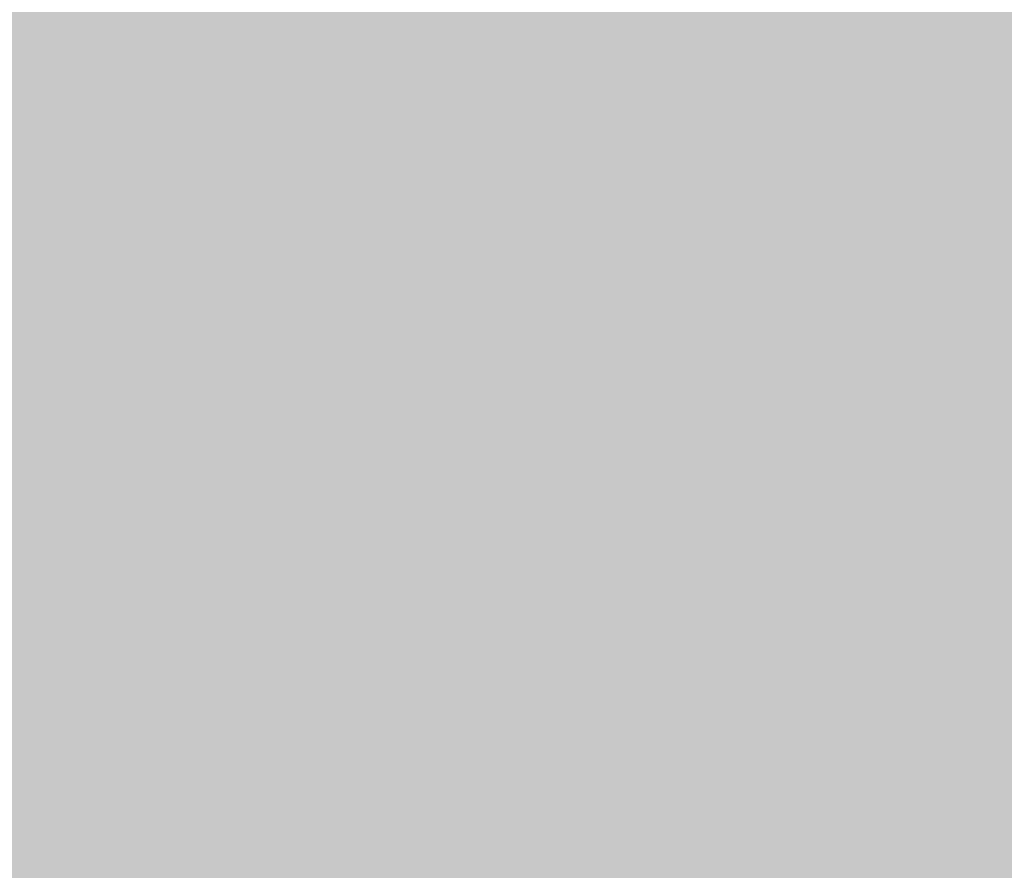
# Model space of a CAD drawing. Units: millimetres. Extents: x -22994 to 29398, y -19990 to 20176.
# Tile 70 of 135: x 225.8137 to 226.3549, y 84.7316 to 85.1994. Entities that reach past the tile are written whole.
import ezdxf
from ezdxf import colors
from ezdxf.entities.mleader import LeaderData, LeaderLine
from ezdxf.math import Vec2, Vec3

# ---------------------------------------------------------------- set-up
doc = ezdxf.new("R2010")
doc.units = ezdxf.units.MM
doc.header["$MEASUREMENT"] = 0
doc.layers.add('M-ANNO-TEXT', color=7, linetype='Continuous', lineweight=25)
doc.layers.add('M-DIMS', color=2, linetype='Continuous', lineweight=18)
doc.styles.get("Standard").update_dxf_attribs({"font": 'arial.ttf'})
doc.dimstyles.get("Standard").update_dxf_attribs({"dimtxt": 0.18, "dimasz": 10000, "dimexe": 0.18, "dimexo": 0.0625, "dimgap": 0.09, "dimtad": 0, "dimtih": 1, "dimtoh": 1, "dimdec": 0, "dimzin": 0, "dimdsep": 46, "dimtxsty": 'Standard', "dimcen": 0.09, "dimadec": 0, "dimazin": 0, "dimtfac": 1, "dimtdec": 0, "dimtofl": 0, "dimtmove": 0, "dimatfit": 3, "dimfxl": 1, "dimtolj": 1, "dimtzin": 0, "dimlwd": 30, "dimarcsym": 0})

# ---------------------------------------------------------------- blocks, each defined once
blk = doc.blocks.new('*D2')
at = {"layer": 'Defpoints', "color": 0, "transparency": 16777216}
for p in [(6.67733, 10.27127), (290.85202, 10.27127), (290.85202, -5.07873)]:
    blk.add_point(p, dxfattribs=at)
at = {"layer": 'M-DIMS', "color": 0, "lineweight": -2, "transparency": 16777216}
for p, q in [((6.67733, 10.20877), (6.67733, -5.25873)), ((290.85202, 10.20877), (290.85202, -5.25873))]:
    blk.add_line(p, q, dxfattribs=at)
at = {"layer": 'M-DIMS', "color": 0, "lineweight": 30, "transparency": 16777216}
for p, q in [((-9993.32267, -5.07873), (-19993.32267, -5.07873)), ((10290.85202, -5.07873), (20290.85202, -5.07873))]:
    blk.add_line(p, q, dxfattribs=at)
at = {"layer": 'M-DIMS', "color": 0, "transparency": 16777216}
for points in [[(-9993.32267, 1661.58794), (-9993.32267, -1671.74539), (6.67733, -5.07873)], [(10290.85202, 1661.58794), (10290.85202, -1671.74539), (290.85202, -5.07873)]]:
    blk.add_solid(points, dxfattribs=at)
at = {"layer": 'M-DIMS', "color": 0, "transparency": 16777216, "insert": (148.76467, -5.07873), "char_height": 0.18, "attachment_point": 5}
blk.add_mtext('\\A1;284.2', dxfattribs=at)
blk = doc.blocks.new('*D3')
at = {"layer": 'Defpoints', "color": 0, "transparency": 16777216}
for p in [(110.26467, 204.16539), (110.26467, 176.36616), (95.83267, 127.96702)]:
    blk.add_point(p, dxfattribs=at)
at = {"layer": 'M-DIMS', "color": 0, "lineweight": -2, "transparency": 16777216}
for p, q in [((95.83267, 128.02952), (95.83267, 204.34539)), ((110.26467, 176.42866), (110.26467, 204.34539))]:
    blk.add_line(p, q, dxfattribs=at)
at = {"layer": 'M-DIMS', "color": 0, "lineweight": 30, "transparency": 16777216}
for p, q in [((-9904.16734, 204.16539), (-19904.16733, 204.16539)), ((10110.26467, 204.16539), (20110.26467, 204.16539))]:
    blk.add_line(p, q, dxfattribs=at)
at = {"layer": 'M-DIMS', "color": 0, "transparency": 16777216}
for points in [[(-9904.16734, 1870.83206), (-9904.16734, -1462.50127), (95.83267, 204.16539)], [(10110.26467, 1870.83206), (10110.26467, -1462.50127), (110.26467, 204.16539)]]:
    blk.add_solid(points, dxfattribs=at)
at = {"layer": 'M-DIMS', "color": 0, "transparency": 16777216, "insert": (103.04867, 204.16539), "char_height": 0.18, "attachment_point": 5}
blk.add_mtext('\\A1;14.432', dxfattribs=at)
blk = doc.blocks.new('*D4')
at = {"layer": 'Defpoints', "color": 0, "transparency": 16777216}
for p in [(116.26467, 204.16539), (110.26467, 176.36616), (116.26467, 176.36616)]:
    blk.add_point(p, dxfattribs=at)
at = {"layer": 'M-DIMS', "color": 0, "lineweight": -2, "transparency": 16777216}
for p, q in [((110.26467, 176.42866), (110.26467, 204.34539)), ((116.26467, 176.42866), (116.26467, 204.34539))]:
    blk.add_line(p, q, dxfattribs=at)
at = {"layer": 'M-DIMS', "color": 0, "lineweight": 30, "transparency": 16777216}
for p, q in [((-9889.73533, 204.16539), (-19889.73533, 204.16539)), ((10116.26467, 204.16539), (20116.26467, 204.16539))]:
    blk.add_line(p, q, dxfattribs=at)
at = {"layer": 'M-DIMS', "color": 0, "transparency": 16777216}
for points in [[(-9889.73533, 1870.83206), (-9889.73533, -1462.50127), (110.26467, 204.16539)], [(10116.26467, 1870.83206), (10116.26467, -1462.50127), (116.26467, 204.16539)]]:
    blk.add_solid(points, dxfattribs=at)
at = {"layer": 'M-DIMS', "color": 0, "transparency": 16777216, "insert": (113.26467, 204.16539), "char_height": 0.18, "attachment_point": 5}
blk.add_mtext('\\A1;6', dxfattribs=at)
blk = doc.blocks.new('*D5')
at = {"layer": 'Defpoints', "color": 0, "transparency": 16777216}
for p in [(181.26467, 204.16539), (116.26467, 176.36616), (181.26467, 176.36616)]:
    blk.add_point(p, dxfattribs=at)
at = {"layer": 'M-DIMS', "color": 0, "lineweight": -2, "transparency": 16777216}
for p, q in [((116.26467, 176.42866), (116.26467, 204.34539)), ((181.26467, 176.42866), (181.26467, 204.34539))]:
    blk.add_line(p, q, dxfattribs=at)
at = {"layer": 'M-DIMS', "color": 0, "lineweight": 30, "transparency": 16777216}
for p, q in [((-9883.73533, 204.16539), (-19883.73533, 204.16539)), ((10181.26467, 204.16539), (20181.26467, 204.16539))]:
    blk.add_line(p, q, dxfattribs=at)
at = {"layer": 'M-DIMS', "color": 0, "transparency": 16777216}
for points in [[(-9883.73533, 1870.83206), (-9883.73533, -1462.50127), (116.26467, 204.16539)], [(10181.26467, 1870.83206), (10181.26467, -1462.50127), (181.26467, 204.16539)]]:
    blk.add_solid(points, dxfattribs=at)
at = {"layer": 'M-DIMS', "color": 0, "transparency": 16777216, "insert": (148.76467, 204.16539), "char_height": 0.18, "attachment_point": 5}
blk.add_mtext('\\A1;65', dxfattribs=at)
blk = doc.blocks.new('*D6')
at = {"layer": 'Defpoints', "color": 0, "transparency": 16777216}
for p in [(187.26467, 204.16539), (181.26467, 176.36616), (187.26467, 176.36616)]:
    blk.add_point(p, dxfattribs=at)
at = {"layer": 'M-DIMS', "color": 0, "lineweight": -2, "transparency": 16777216}
for p, q in [((181.26467, 176.42866), (181.26467, 204.34539)), ((187.26467, 176.42866), (187.26467, 204.34539))]:
    blk.add_line(p, q, dxfattribs=at)
at = {"layer": 'M-DIMS', "color": 0, "lineweight": 30, "transparency": 16777216}
for p, q in [((-9818.73533, 204.16539), (-19818.73533, 204.16539)), ((10187.26467, 204.16539), (20187.26467, 204.16539))]:
    blk.add_line(p, q, dxfattribs=at)
at = {"layer": 'M-DIMS', "color": 0, "transparency": 16777216}
for points in [[(-9818.73533, 1870.83206), (-9818.73533, -1462.50127), (181.26467, 204.16539)], [(10187.26467, 1870.83206), (10187.26467, -1462.50127), (187.26467, 204.16539)]]:
    blk.add_solid(points, dxfattribs=at)
at = {"layer": 'M-DIMS', "color": 0, "transparency": 16777216, "insert": (184.26467, 204.16539), "char_height": 0.18, "attachment_point": 5}
blk.add_mtext('\\A1;6', dxfattribs=at)
blk = doc.blocks.new('*D7')
at = {"layer": 'Defpoints', "color": 0, "transparency": 16777216}
for p in [(201.69668, 204.16539), (187.26467, 176.36616), (201.69668, 127.96702)]:
    blk.add_point(p, dxfattribs=at)
at = {"layer": 'M-DIMS', "color": 0, "lineweight": -2, "transparency": 16777216}
for p, q in [((187.26467, 176.42866), (187.26467, 204.34539)), ((201.69668, 128.02952), (201.69668, 204.34539))]:
    blk.add_line(p, q, dxfattribs=at)
at = {"layer": 'M-DIMS', "color": 0, "lineweight": 30, "transparency": 16777216}
for p, q in [((-9812.73533, 204.16539), (-19812.73533, 204.16539)), ((10201.69668, 204.16539), (20201.69668, 204.16539))]:
    blk.add_line(p, q, dxfattribs=at)
at = {"layer": 'M-DIMS', "color": 0, "transparency": 16777216}
for points in [[(-9812.73533, 1870.83206), (-9812.73533, -1462.50127), (187.26467, 204.16539)], [(10201.69668, 1870.83206), (10201.69668, -1462.50127), (201.69668, 204.16539)]]:
    blk.add_solid(points, dxfattribs=at)
at = {"layer": 'M-DIMS', "color": 0, "transparency": 16777216, "insert": (194.48068, 204.16539), "char_height": 0.18, "attachment_point": 5}
blk.add_mtext('\\A1;14.432', dxfattribs=at)
blk = doc.blocks.new('*D8')
at = {"layer": 'Defpoints', "color": 0, "transparency": 16777216}
for p in [(227.64848, 204.16539), (227.64848, 146.72957), (201.69668, 127.96702)]:
    blk.add_point(p, dxfattribs=at)
at = {"layer": 'M-DIMS', "color": 0, "lineweight": -2, "transparency": 16777216}
for p, q in [((201.69668, 128.02952), (201.69668, 204.34539)), ((227.64848, 146.79207), (227.64848, 204.34539))]:
    blk.add_line(p, q, dxfattribs=at)
at = {"layer": 'M-DIMS', "color": 0, "lineweight": 30, "transparency": 16777216}
for p, q in [((-9798.30332, 204.16539), (-19798.30332, 204.16539)), ((10227.64848, 204.16539), (20227.64848, 204.16539))]:
    blk.add_line(p, q, dxfattribs=at)
at = {"layer": 'M-DIMS', "color": 0, "transparency": 16777216}
for points in [[(-9798.30332, 1870.83206), (-9798.30332, -1462.50127), (201.69668, 204.16539)], [(10227.64848, 1870.83206), (10227.64848, -1462.50127), (227.64848, 204.16539)]]:
    blk.add_solid(points, dxfattribs=at)
at = {"layer": 'M-DIMS', "color": 0, "transparency": 16777216, "insert": (214.67258, 204.16539), "char_height": 0.18, "attachment_point": 5}
blk.add_mtext('\\A1;25.95', dxfattribs=at)
blk = doc.blocks.new('*D9')
at = {"layer": 'Defpoints', "color": 0, "transparency": 16777216}
for p in [(187.26467, 176.36616), (306.20202, 176.36616), (290.85202, 10.27127)]:
    blk.add_point(p, dxfattribs=at)
at = {"layer": 'M-DIMS', "color": 0, "lineweight": 30, "transparency": 16777216}
for p, q in [((306.20202, 10176.36616), (306.20202, 20176.36616)), ((306.20202, -9989.72873), (306.20202, -19989.72873))]:
    blk.add_line(p, q, dxfattribs=at)
at = {"layer": 'M-DIMS', "color": 0, "lineweight": -2, "transparency": 16777216}
for p, q in [((187.32717, 176.36616), (306.38202, 176.36616)), ((290.91452, 10.27127), (306.38202, 10.27127))]:
    blk.add_line(p, q, dxfattribs=at)
at = {"layer": 'M-DIMS', "color": 0, "transparency": 16777216}
for points in [[(-1360.46465, 10176.36616), (1972.86869, 10176.36616), (306.20202, 176.36616)], [(-1360.46465, -9989.72873), (1972.86869, -9989.72873), (306.20202, 10.27127)]]:
    blk.add_solid(points, dxfattribs=at)
at = {"layer": 'M-DIMS', "color": 0, "transparency": 16777216, "insert": (306.20202, 93.31872), "char_height": 0.18, "attachment_point": 5}
blk.add_mtext('\\A1;166.1', dxfattribs=at)
blk = doc.blocks.new('*D10')
at = {"layer": 'Defpoints', "color": 0, "transparency": 16777216}
for p in [(125.64978, 136.0713), (133.34587, 136.0713), (133.34587, -5.07873)]:
    blk.add_point(p, dxfattribs=at)
at = {"layer": 'M-DIMS', "color": 0, "lineweight": -2, "transparency": 16777216}
for p, q in [((125.64978, 136.0088), (125.64978, -5.25872)), ((133.34587, 136.0088), (133.34587, -5.25872))]:
    blk.add_line(p, q, dxfattribs=at)
at = {"layer": 'M-DIMS', "color": 0, "lineweight": 30, "transparency": 16777216}
for p, q in [((-9874.35022, -5.07873), (-19874.35022, -5.07873)), ((10133.34587, -5.07873), (20133.34587, -5.07873))]:
    blk.add_line(p, q, dxfattribs=at)
at = {"layer": 'M-DIMS', "color": 0, "transparency": 16777216}
for points in [[(-9874.35022, 1661.58794), (-9874.35022, -1671.74539), (125.64978, -5.07873)], [(10133.34587, 1661.58794), (10133.34587, -1671.74539), (133.34587, -5.07873)]]:
    blk.add_solid(points, dxfattribs=at)
at = {"layer": 'M-DIMS', "color": 0, "transparency": 16777216, "insert": (129.49783, -5.07873), "char_height": 0.18, "attachment_point": 5}
blk.add_mtext('\\A1;7.696', dxfattribs=at)
blk = doc.blocks.new('*D11')
at = {"layer": 'Defpoints', "color": 0, "transparency": 16777216}
for p in [(133.34587, 136.0713), (135.64978, 136.0713), (135.64978, -5.07873)]:
    blk.add_point(p, dxfattribs=at)
at = {"layer": 'M-DIMS', "color": 0, "lineweight": -2, "transparency": 16777216}
for p, q in [((133.34587, 136.0088), (133.34587, -5.25872)), ((135.64978, 136.0088), (135.64978, -5.25872))]:
    blk.add_line(p, q, dxfattribs=at)
at = {"layer": 'M-DIMS', "color": 0, "lineweight": 30, "transparency": 16777216}
for p, q in [((-9866.65413, -5.07873), (-19866.65413, -5.07873)), ((10135.64978, -5.07873), (20135.64978, -5.07873))]:
    blk.add_line(p, q, dxfattribs=at)
at = {"layer": 'M-DIMS', "color": 0, "transparency": 16777216}
for points in [[(-9866.65413, 1661.58794), (-9866.65413, -1671.74539), (133.34587, -5.07873)], [(10135.64978, 1661.58794), (10135.64978, -1671.74539), (135.64978, -5.07873)]]:
    blk.add_solid(points, dxfattribs=at)
at = {"layer": 'M-DIMS', "color": 0, "transparency": 16777216, "insert": (134.49783, -5.07873), "char_height": 0.18, "attachment_point": 5}
blk.add_mtext('\\A1;2.304', dxfattribs=at)
blk = doc.blocks.new('*D12')
at = {"layer": 'Defpoints', "color": 0, "transparency": 16777216}
for p in [(135.64978, 136.0713), (145.64978, 136.0713), (145.64978, -5.07873)]:
    blk.add_point(p, dxfattribs=at)
at = {"layer": 'M-DIMS', "color": 0, "lineweight": -2, "transparency": 16777216}
for p, q in [((135.64978, 136.0088), (135.64978, -5.25872)), ((145.64978, 136.0088), (145.64978, -5.25872))]:
    blk.add_line(p, q, dxfattribs=at)
at = {"layer": 'M-DIMS', "color": 0, "lineweight": 30, "transparency": 16777216}
for p, q in [((-9864.35022, -5.07873), (-19864.35022, -5.07873)), ((10145.64978, -5.07873), (20145.64978, -5.07873))]:
    blk.add_line(p, q, dxfattribs=at)
at = {"layer": 'M-DIMS', "color": 0, "transparency": 16777216}
for points in [[(-9864.35022, 1661.58794), (-9864.35022, -1671.74539), (135.64978, -5.07873)], [(10145.64978, 1661.58794), (10145.64978, -1671.74539), (145.64978, -5.07873)]]:
    blk.add_solid(points, dxfattribs=at)
at = {"layer": 'M-DIMS', "color": 0, "transparency": 16777216, "insert": (140.64978, -5.07873), "char_height": 0.18, "attachment_point": 5}
blk.add_mtext('\\A1;10', dxfattribs=at)
blk = doc.blocks.new('*D13')
at = {"layer": 'Defpoints', "color": 0, "transparency": 16777216}
for p in [(145.64978, 136.0713), (155.64978, 136.0713), (155.64978, -5.07873)]:
    blk.add_point(p, dxfattribs=at)
at = {"layer": 'M-DIMS', "color": 0, "lineweight": -2, "transparency": 16777216}
for p, q in [((145.64978, 136.0088), (145.64978, -5.25872)), ((155.64978, 136.0088), (155.64978, -5.25872))]:
    blk.add_line(p, q, dxfattribs=at)
at = {"layer": 'M-DIMS', "color": 0, "lineweight": 30, "transparency": 16777216}
for p, q in [((-9854.35022, -5.07873), (-19854.35022, -5.07873)), ((10155.64978, -5.07873), (20155.64978, -5.07873))]:
    blk.add_line(p, q, dxfattribs=at)
at = {"layer": 'M-DIMS', "color": 0, "transparency": 16777216}
for points in [[(-9854.35022, 1661.58794), (-9854.35022, -1671.74539), (145.64978, -5.07873)], [(10155.64978, 1661.58794), (10155.64978, -1671.74539), (155.64978, -5.07873)]]:
    blk.add_solid(points, dxfattribs=at)
at = {"layer": 'M-DIMS', "color": 0, "transparency": 16777216, "insert": (150.64978, -5.07873), "char_height": 0.18, "attachment_point": 5}
blk.add_mtext('\\A1;10', dxfattribs=at)
blk = doc.blocks.new('*D14')
at = {"layer": 'Defpoints', "color": 0, "transparency": 16777216}
for p in [(155.64978, 136.0713), (165.64978, 136.0713), (165.64978, -5.07873)]:
    blk.add_point(p, dxfattribs=at)
at = {"layer": 'M-DIMS', "color": 0, "lineweight": -2, "transparency": 16777216}
for p, q in [((155.64978, 136.0088), (155.64978, -5.25872)), ((165.64978, 136.0088), (165.64978, -5.25872))]:
    blk.add_line(p, q, dxfattribs=at)
at = {"layer": 'M-DIMS', "color": 0, "lineweight": 30, "transparency": 16777216}
for p, q in [((-9844.35022, -5.07873), (-19844.35022, -5.07873)), ((10165.64978, -5.07873), (20165.64978, -5.07873))]:
    blk.add_line(p, q, dxfattribs=at)
at = {"layer": 'M-DIMS', "color": 0, "transparency": 16777216}
for points in [[(-9844.35022, 1661.58794), (-9844.35022, -1671.74539), (155.64978, -5.07873)], [(10165.64978, 1661.58794), (10165.64978, -1671.74539), (165.64978, -5.07873)]]:
    blk.add_solid(points, dxfattribs=at)
at = {"layer": 'M-DIMS', "color": 0, "transparency": 16777216, "insert": (160.64978, -5.07873), "char_height": 0.18, "attachment_point": 5}
blk.add_mtext('\\A1;10', dxfattribs=at)
blk = doc.blocks.new('*D15')
at = {"layer": 'Defpoints', "color": 0, "transparency": 16777216}
for p in [(173.34587, 154.78801), (173.34587, 136.0713), (306.20202, 136.0713)]:
    blk.add_point(p, dxfattribs=at)
at = {"layer": 'M-DIMS', "color": 0, "lineweight": 30, "transparency": 16777216}
for p, q in [((306.20202, 10154.78801), (306.20202, 20154.78801)), ((306.20202, -9863.9287), (306.20202, -19863.9287))]:
    blk.add_line(p, q, dxfattribs=at)
at = {"layer": 'M-DIMS', "color": 0, "lineweight": -2, "transparency": 16777216}
for p, q in [((173.40837, 154.78801), (306.38202, 154.78801)), ((173.40837, 136.0713), (306.38202, 136.0713))]:
    blk.add_line(p, q, dxfattribs=at)
at = {"layer": 'M-DIMS', "color": 0, "transparency": 16777216}
for points in [[(-1360.46465, 10154.78801), (1972.86869, 10154.78801), (306.20202, 154.78801)], [(-1360.46465, -9863.9287), (1972.86869, -9863.9287), (306.20202, 136.0713)]]:
    blk.add_solid(points, dxfattribs=at)
at = {"layer": 'M-DIMS', "color": 0, "transparency": 16777216, "insert": (306.20202, 145.42965), "char_height": 0.18, "attachment_point": 5}
blk.add_mtext('\\A1;18.717', dxfattribs=at)
blk = doc.blocks.new('*D16')
at = {"layer": 'Defpoints', "color": 0, "transparency": 16777216}
for p in [(120.17023, 204.16539), (110.46575, 48.03494), (120.17023, 48.03494)]:
    blk.add_point(p, dxfattribs=at)
at = {"layer": 'M-DIMS', "color": 0, "lineweight": -2, "transparency": 16777216}
for p, q in [((110.46575, 48.09744), (110.46575, 204.34539)), ((120.17023, 48.09744), (120.17023, 204.34539))]:
    blk.add_line(p, q, dxfattribs=at)
at = {"layer": 'M-DIMS', "color": 0, "lineweight": 30, "transparency": 16777216}
for p, q in [((-9889.53425, 204.16539), (-19889.53425, 204.16539)), ((10120.17023, 204.16539), (20120.17023, 204.16539))]:
    blk.add_line(p, q, dxfattribs=at)
at = {"layer": 'M-DIMS', "color": 0, "transparency": 16777216}
for points in [[(-9889.53425, 1870.83206), (-9889.53425, -1462.50127), (110.46575, 204.16539)], [(10120.17023, 1870.83206), (10120.17023, -1462.50127), (120.17023, 204.16539)]]:
    blk.add_solid(points, dxfattribs=at)
at = {"layer": 'M-DIMS', "color": 0, "transparency": 16777216, "insert": (115.31799, 204.16539), "char_height": 0.18, "attachment_point": 5}
blk.add_mtext('\\A1;9.704', dxfattribs=at)
blk = doc.blocks.new('*D17')
at = {"layer": 'Defpoints', "color": 0, "transparency": 16777216}
for p in [(126.17023, 204.16539), (120.17023, 48.03494), (126.17023, 48.03494)]:
    blk.add_point(p, dxfattribs=at)
at = {"layer": 'M-DIMS', "color": 0, "lineweight": -2, "transparency": 16777216}
for p, q in [((120.17023, 48.09744), (120.17023, 204.34539)), ((126.17023, 48.09744), (126.17023, 204.34539))]:
    blk.add_line(p, q, dxfattribs=at)
at = {"layer": 'M-DIMS', "color": 0, "lineweight": 30, "transparency": 16777216}
for p, q in [((-9879.82977, 204.16539), (-19879.82977, 204.16539)), ((10126.17023, 204.16539), (20126.17023, 204.16539))]:
    blk.add_line(p, q, dxfattribs=at)
at = {"layer": 'M-DIMS', "color": 0, "transparency": 16777216}
for points in [[(-9879.82977, 1870.83206), (-9879.82977, -1462.50127), (120.17023, 204.16539)], [(10126.17023, 1870.83206), (10126.17023, -1462.50127), (126.17023, 204.16539)]]:
    blk.add_solid(points, dxfattribs=at)
at = {"layer": 'M-DIMS', "color": 0, "transparency": 16777216, "insert": (123.17023, 204.16539), "char_height": 0.18, "attachment_point": 5}
blk.add_mtext('\\A1;6', dxfattribs=at)
blk = doc.blocks.new('*D18')
at = {"layer": 'Defpoints', "color": 0, "transparency": 16777216}
for p in [(132.17023, 204.16539), (126.17023, 48.03494), (132.17023, 48.03494)]:
    blk.add_point(p, dxfattribs=at)
at = {"layer": 'M-DIMS', "color": 0, "lineweight": -2, "transparency": 16777216}
for p, q in [((126.17023, 48.09744), (126.17023, 204.34539)), ((132.17023, 48.09744), (132.17023, 204.34539))]:
    blk.add_line(p, q, dxfattribs=at)
at = {"layer": 'M-DIMS', "color": 0, "lineweight": 30, "transparency": 16777216}
for p, q in [((-9873.82977, 204.16539), (-19873.82977, 204.16539)), ((10132.17023, 204.16539), (20132.17023, 204.16539))]:
    blk.add_line(p, q, dxfattribs=at)
at = {"layer": 'M-DIMS', "color": 0, "transparency": 16777216}
for points in [[(-9873.82977, 1870.83206), (-9873.82977, -1462.50127), (126.17023, 204.16539)], [(10132.17023, 1870.83206), (10132.17023, -1462.50127), (132.17023, 204.16539)]]:
    blk.add_solid(points, dxfattribs=at)
at = {"layer": 'M-DIMS', "color": 0, "transparency": 16777216, "insert": (129.17023, 204.16539), "char_height": 0.18, "attachment_point": 5}
blk.add_mtext('\\A1;6', dxfattribs=at)
blk = doc.blocks.new('*D19')
at = {"layer": 'Defpoints', "color": 0, "transparency": 16777216}
for p in [(138.17023, 204.16539), (132.17023, 48.03494), (138.17023, 48.03494)]:
    blk.add_point(p, dxfattribs=at)
at = {"layer": 'M-DIMS', "color": 0, "lineweight": -2, "transparency": 16777216}
for p, q in [((132.17023, 48.09744), (132.17023, 204.34539)), ((138.17023, 48.09744), (138.17023, 204.34539))]:
    blk.add_line(p, q, dxfattribs=at)
at = {"layer": 'M-DIMS', "color": 0, "lineweight": 30, "transparency": 16777216}
for p, q in [((-9867.82977, 204.16539), (-19867.82977, 204.16539)), ((10138.17023, 204.16539), (20138.17023, 204.16539))]:
    blk.add_line(p, q, dxfattribs=at)
at = {"layer": 'M-DIMS', "color": 0, "transparency": 16777216}
for points in [[(-9867.82977, 1870.83206), (-9867.82977, -1462.50127), (132.17023, 204.16539)], [(10138.17023, 1870.83206), (10138.17023, -1462.50127), (138.17023, 204.16539)]]:
    blk.add_solid(points, dxfattribs=at)
at = {"layer": 'M-DIMS', "color": 0, "transparency": 16777216, "insert": (135.17023, 204.16539), "char_height": 0.18, "attachment_point": 5}
blk.add_mtext('\\A1;6', dxfattribs=at)
blk = doc.blocks.new('*D20')
at = {"layer": 'Defpoints', "color": 0, "transparency": 16777216}
for p in [(144.17023, 204.16539), (138.17023, 48.03494), (144.17023, 48.03494)]:
    blk.add_point(p, dxfattribs=at)
at = {"layer": 'M-DIMS', "color": 0, "lineweight": -2, "transparency": 16777216}
for p, q in [((138.17023, 48.09744), (138.17023, 204.34539)), ((144.17023, 48.09744), (144.17023, 204.34539))]:
    blk.add_line(p, q, dxfattribs=at)
at = {"layer": 'M-DIMS', "color": 0, "lineweight": 30, "transparency": 16777216}
for p, q in [((-9861.82977, 204.16539), (-19861.82977, 204.16539)), ((10144.17023, 204.16539), (20144.17023, 204.16539))]:
    blk.add_line(p, q, dxfattribs=at)
at = {"layer": 'M-DIMS', "color": 0, "transparency": 16777216}
for points in [[(-9861.82977, 1870.83206), (-9861.82977, -1462.50127), (138.17023, 204.16539)], [(10144.17023, 1870.83206), (10144.17023, -1462.50127), (144.17023, 204.16539)]]:
    blk.add_solid(points, dxfattribs=at)
at = {"layer": 'M-DIMS', "color": 0, "transparency": 16777216, "insert": (141.17023, 204.16539), "char_height": 0.18, "attachment_point": 5}
blk.add_mtext('\\A1;6', dxfattribs=at)
blk = doc.blocks.new('*D21')
at = {"layer": 'Defpoints', "color": 0, "transparency": 16777216}
for p in [(149.11567, 204.16539), (144.17023, 48.03494), (149.11567, 48.03494)]:
    blk.add_point(p, dxfattribs=at)
at = {"layer": 'M-DIMS', "color": 0, "lineweight": -2, "transparency": 16777216}
for p, q in [((144.17023, 48.09744), (144.17023, 204.34539)), ((149.11567, 48.09744), (149.11567, 204.34539))]:
    blk.add_line(p, q, dxfattribs=at)
at = {"layer": 'M-DIMS', "color": 0, "lineweight": 30, "transparency": 16777216}
for p, q in [((-9855.82977, 204.16539), (-19855.82977, 204.16539)), ((10149.11567, 204.16539), (20149.11567, 204.16539))]:
    blk.add_line(p, q, dxfattribs=at)
at = {"layer": 'M-DIMS', "color": 0, "transparency": 16777216}
for points in [[(-9855.82977, 1870.83206), (-9855.82977, -1462.50127), (144.17023, 204.16539)], [(10149.11567, 1870.83206), (10149.11567, -1462.50127), (149.11567, 204.16539)]]:
    blk.add_solid(points, dxfattribs=at)
at = {"layer": 'M-DIMS', "color": 0, "transparency": 16777216, "insert": (146.64295, 204.16539), "char_height": 0.18, "attachment_point": 5}
blk.add_mtext('\\A1;4.945', dxfattribs=at)
blk = doc.blocks.new('*D22')
at = {"layer": 'Defpoints', "color": 0, "transparency": 16777216}
for p in [(149.11567, 30.98952), (155.11567, 30.98952), (155.11567, -5.07873)]:
    blk.add_point(p, dxfattribs=at)
at = {"layer": 'M-DIMS', "color": 0, "lineweight": -2, "transparency": 16777216}
for p, q in [((149.11567, 30.92702), (149.11567, -5.25872)), ((155.11567, 30.92702), (155.11567, -5.25872))]:
    blk.add_line(p, q, dxfattribs=at)
at = {"layer": 'M-DIMS', "color": 0, "lineweight": 30, "transparency": 16777216}
for p, q in [((-9850.88433, -5.07873), (-19850.88433, -5.07873)), ((10155.11567, -5.07873), (20155.11567, -5.07873))]:
    blk.add_line(p, q, dxfattribs=at)
at = {"layer": 'M-DIMS', "color": 0, "transparency": 16777216}
for points in [[(-9850.88433, 1661.58794), (-9850.88433, -1671.74539), (149.11567, -5.07873)], [(10155.11567, 1661.58794), (10155.11567, -1671.74539), (155.11567, -5.07873)]]:
    blk.add_solid(points, dxfattribs=at)
at = {"layer": 'M-DIMS', "color": 0, "transparency": 16777216, "insert": (152.11567, -5.07873), "char_height": 0.18, "attachment_point": 5}
blk.add_mtext('\\A1;6', dxfattribs=at)
blk = doc.blocks.new('*D23')
at = {"layer": 'Defpoints', "color": 0, "transparency": 16777216}
for p in [(155.11567, 30.98952), (161.11567, 30.98952), (161.11567, -5.07873)]:
    blk.add_point(p, dxfattribs=at)
at = {"layer": 'M-DIMS', "color": 0, "lineweight": -2, "transparency": 16777216}
for p, q in [((155.11567, 30.92702), (155.11567, -5.25872)), ((161.11567, 30.92702), (161.11567, -5.25872))]:
    blk.add_line(p, q, dxfattribs=at)
at = {"layer": 'M-DIMS', "color": 0, "lineweight": 30, "transparency": 16777216}
for p, q in [((-9844.88433, -5.07873), (-19844.88433, -5.07873)), ((10161.11567, -5.07873), (20161.11567, -5.07873))]:
    blk.add_line(p, q, dxfattribs=at)
at = {"layer": 'M-DIMS', "color": 0, "transparency": 16777216}
for points in [[(-9844.88433, 1661.58794), (-9844.88433, -1671.74539), (155.11567, -5.07873)], [(10161.11567, 1661.58794), (10161.11567, -1671.74539), (161.11567, -5.07873)]]:
    blk.add_solid(points, dxfattribs=at)
at = {"layer": 'M-DIMS', "color": 0, "transparency": 16777216, "insert": (158.11567, -5.07873), "char_height": 0.18, "attachment_point": 5}
blk.add_mtext('\\A1;6', dxfattribs=at)
blk = doc.blocks.new('*D24')
at = {"layer": 'Defpoints', "color": 0, "transparency": 16777216}
for p in [(161.11567, 30.98952), (166.43874, 30.98952), (166.43874, -5.07873)]:
    blk.add_point(p, dxfattribs=at)
at = {"layer": 'M-DIMS', "color": 0, "lineweight": -2, "transparency": 16777216}
for p, q in [((161.11567, 30.92702), (161.11567, -5.25872)), ((166.43874, 30.92702), (166.43874, -5.25872))]:
    blk.add_line(p, q, dxfattribs=at)
at = {"layer": 'M-DIMS', "color": 0, "lineweight": 30, "transparency": 16777216}
for p, q in [((-9838.88433, -5.07873), (-19838.88433, -5.07873)), ((10166.43874, -5.07873), (20166.43874, -5.07873))]:
    blk.add_line(p, q, dxfattribs=at)
at = {"layer": 'M-DIMS', "color": 0, "transparency": 16777216}
for points in [[(-9838.88433, 1661.58794), (-9838.88433, -1671.74539), (161.11567, -5.07873)], [(10166.43874, 1661.58794), (10166.43874, -1671.74539), (166.43874, -5.07873)]]:
    blk.add_solid(points, dxfattribs=at)
at = {"layer": 'M-DIMS', "color": 0, "transparency": 16777216, "insert": (163.7772, -5.07873), "char_height": 0.18, "attachment_point": 5}
blk.add_mtext('\\A1;5.323', dxfattribs=at)
blk = doc.blocks.new('*D25')
at = {"layer": 'Defpoints', "color": 0, "transparency": 16777216}
for p in [(166.43874, 30.98952), (172.43874, 30.98952), (172.43874, -5.07873)]:
    blk.add_point(p, dxfattribs=at)
at = {"layer": 'M-DIMS', "color": 0, "lineweight": -2, "transparency": 16777216}
for p, q in [((166.43874, 30.92702), (166.43874, -5.25872)), ((172.43874, 30.92702), (172.43874, -5.25872))]:
    blk.add_line(p, q, dxfattribs=at)
at = {"layer": 'M-DIMS', "color": 0, "lineweight": 30, "transparency": 16777216}
for p, q in [((-9833.56126, -5.07873), (-19833.56126, -5.07873)), ((10172.43874, -5.07873), (20172.43874, -5.07873))]:
    blk.add_line(p, q, dxfattribs=at)
at = {"layer": 'M-DIMS', "color": 0, "transparency": 16777216}
for points in [[(-9833.56126, 1661.58794), (-9833.56126, -1671.74539), (166.43874, -5.07873)], [(10172.43874, 1661.58794), (10172.43874, -1671.74539), (172.43874, -5.07873)]]:
    blk.add_solid(points, dxfattribs=at)
at = {"layer": 'M-DIMS', "color": 0, "transparency": 16777216, "insert": (169.43874, -5.07873), "char_height": 0.18, "attachment_point": 5}
blk.add_mtext('\\A1;6', dxfattribs=at)
blk = doc.blocks.new('*D26')
at = {"layer": 'Defpoints', "color": 0, "transparency": 16777216}
for p in [(172.43874, 30.98952), (178.43874, 30.98952), (178.43874, -5.07873)]:
    blk.add_point(p, dxfattribs=at)
at = {"layer": 'M-DIMS', "color": 0, "lineweight": -2, "transparency": 16777216}
for p, q in [((172.43874, 30.92702), (172.43874, -5.25872)), ((178.43874, 30.92702), (178.43874, -5.25872))]:
    blk.add_line(p, q, dxfattribs=at)
at = {"layer": 'M-DIMS', "color": 0, "lineweight": 30, "transparency": 16777216}
for p, q in [((-9827.56126, -5.07873), (-19827.56126, -5.07873)), ((10178.43874, -5.07873), (20178.43874, -5.07873))]:
    blk.add_line(p, q, dxfattribs=at)
at = {"layer": 'M-DIMS', "color": 0, "transparency": 16777216}
for points in [[(-9827.56126, 1661.58794), (-9827.56126, -1671.74539), (172.43874, -5.07873)], [(10178.43874, 1661.58794), (10178.43874, -1671.74539), (178.43874, -5.07873)]]:
    blk.add_solid(points, dxfattribs=at)
at = {"layer": 'M-DIMS', "color": 0, "transparency": 16777216, "insert": (175.43874, -5.07873), "char_height": 0.18, "attachment_point": 5}
blk.add_mtext('\\A1;6', dxfattribs=at)
blk = doc.blocks.new('*D27')
at = {"layer": 'Defpoints', "color": 0, "transparency": 16777216}
for p in [(178.43874, 30.98952), (188.11747, 30.98952), (188.11747, -5.07873)]:
    blk.add_point(p, dxfattribs=at)
at = {"layer": 'M-DIMS', "color": 0, "lineweight": -2, "transparency": 16777216}
for p, q in [((178.43874, 30.92702), (178.43874, -5.25872)), ((188.11747, 30.92702), (188.11747, -5.25872))]:
    blk.add_line(p, q, dxfattribs=at)
at = {"layer": 'M-DIMS', "color": 0, "lineweight": 30, "transparency": 16777216}
for p, q in [((-9821.56126, -5.07873), (-19821.56126, -5.07873)), ((10188.11747, -5.07873), (20188.11747, -5.07873))]:
    blk.add_line(p, q, dxfattribs=at)
at = {"layer": 'M-DIMS', "color": 0, "transparency": 16777216}
for points in [[(-9821.56126, 1661.58794), (-9821.56126, -1671.74539), (178.43874, -5.07873)], [(10188.11747, 1661.58794), (10188.11747, -1671.74539), (188.11747, -5.07873)]]:
    blk.add_solid(points, dxfattribs=at)
at = {"layer": 'M-DIMS', "color": 0, "transparency": 16777216, "insert": (183.27811, -5.07873), "char_height": 0.18, "attachment_point": 5}
blk.add_mtext('\\A1;9.679', dxfattribs=at)
blk = doc.blocks.new('*D28')
at = {"layer": 'Defpoints', "color": 0, "transparency": 16777216}
for p in [(188.11747, 48.03494), (306.20202, 48.03494), (188.11747, 30.98952)]:
    blk.add_point(p, dxfattribs=at)
at = {"layer": 'M-DIMS', "color": 0, "lineweight": 30, "transparency": 16777216}
for p, q in [((306.20202, 10048.03494), (306.20202, 20048.03494)), ((306.20202, -9969.01048), (306.20202, -19969.01048))]:
    blk.add_line(p, q, dxfattribs=at)
at = {"layer": 'M-DIMS', "color": 0, "lineweight": -2, "transparency": 16777216}
for p, q in [((188.17997, 48.03494), (306.38202, 48.03494)), ((188.17997, 30.98952), (306.38202, 30.98952))]:
    blk.add_line(p, q, dxfattribs=at)
at = {"layer": 'M-DIMS', "color": 0, "transparency": 16777216}
for points in [[(-1360.46465, 10048.03494), (1972.86869, 10048.03494), (306.20202, 48.03494)], [(-1360.46465, -9969.01048), (1972.86869, -9969.01048), (306.20202, 30.98952)]]:
    blk.add_solid(points, dxfattribs=at)
at = {"layer": 'M-DIMS', "color": 0, "transparency": 16777216, "insert": (306.20202, 39.51223), "char_height": 0.18, "attachment_point": 5}
blk.add_mtext('\\A1;17.045', dxfattribs=at)
blk = doc.blocks.new('*D29')
at = {"layer": 'Defpoints', "color": 0, "transparency": 16777216}
for p in [(36.80064, 80.04502), (64.02964, 80.045)]:
    blk.add_point(p, dxfattribs=at)
at = {"layer": 'M-DIMS', "color": 0, "lineweight": -2, "transparency": 16777216}
for p, q in [((50.41514, 79.95501), (50.41514, 80.13501)), ((50.32514, 80.04501), (50.50514, 80.04501))]:
    blk.add_line(p, q, dxfattribs=at)
at = {"layer": 'M-DIMS', "color": 0, "lineweight": 30, "transparency": 16777216}
blk.add_line((20064.02964, 80.03031), (10064.02964, 80.03765), dxfattribs=at)
at = {"layer": 'M-DIMS', "color": 0, "transparency": 16777216}
blk.add_solid([(10064.03087, 1746.70432), (10064.02842, -1586.62901), (64.02964, 80.045)], dxfattribs=at)
at = {"layer": 'M-DIMS', "color": 0, "transparency": 16777216, "insert": (20064.52126, 80.03031), "char_height": 0.18, "attachment_point": 5}
blk.add_mtext('\\A1;∅27.23', dxfattribs=at)
blk = doc.blocks.new('*D30')
at = {"layer": 'Defpoints', "color": 0, "transparency": 16777216}
for p in [(216.31485, 146.72913), (238.98211, 146.73)]:
    blk.add_point(p, dxfattribs=at)
at = {"layer": 'M-DIMS', "color": 0, "lineweight": 30, "transparency": 16777216}
blk.add_line((20238.9821, 147.49586), (10238.98211, 147.11293), dxfattribs=at)
at = {"layer": 'M-DIMS', "color": 0, "lineweight": -2, "transparency": 16777216}
for p, q in [((227.64848, 146.63957), (227.64848, 146.81957)), ((227.55848, 146.72957), (227.73848, 146.72957))]:
    blk.add_line(p, q, dxfattribs=at)
at = {"layer": 'M-DIMS', "color": 0, "transparency": 16777216}
blk.add_solid([(10238.91828, 1813.7796), (10239.04593, -1519.55373), (238.98211, 146.73)], dxfattribs=at)
at = {"layer": 'M-DIMS', "color": 0, "transparency": 16777216, "insert": (20239.54365, 147.49586), "char_height": 0.18, "attachment_point": 5}
blk.add_mtext('\\A1;∅22.667', dxfattribs=at)
blk = doc.blocks.new('*D31')
at = {"layer": 'Defpoints', "color": 0, "transparency": 16777216}
for p in [(223.16413, 146.72913), (232.13283, 146.73)]:
    blk.add_point(p, dxfattribs=at)
at = {"layer": 'M-DIMS', "color": 0, "lineweight": 30, "transparency": 16777216}
blk.add_line((20232.13273, 148.66562), (10232.13278, 147.69781), dxfattribs=at)
at = {"layer": 'M-DIMS', "color": 0, "lineweight": -2, "transparency": 16777216}
for p, q in [((227.64848, 146.63957), (227.64848, 146.81957)), ((227.55848, 146.72957), (227.73848, 146.72957))]:
    blk.add_line(p, q, dxfattribs=at)
at = {"layer": 'M-DIMS', "color": 0, "transparency": 16777216}
blk.add_solid([(10231.97148, 1814.36447), (10232.29408, -1518.96885), (232.13283, 146.73)], dxfattribs=at)
at = {"layer": 'M-DIMS', "color": 0, "transparency": 16777216, "insert": (20232.62454, 148.66562), "char_height": 0.18, "attachment_point": 5}
blk.add_mtext('\\A1;∅8.969', dxfattribs=at)
blk = doc.blocks.new('*D36')
at = {"layer": 'Defpoints', "color": 0, "transparency": 16777216}
for p in [(46.39, 31.30349), (46.38747, 26.59341)]:
    blk.add_point(p, dxfattribs=at)
at = {"layer": 'M-DIMS', "color": 0, "lineweight": 30, "transparency": 16777216}
for p, q in [((57.1499, 20031.3006), (51.76995, 10031.30205)), ((10057.1499, 20031.3006), (57.1499, 20031.3006))]:
    blk.add_line(p, q, dxfattribs=at)
at = {"layer": 'M-DIMS', "color": 0, "lineweight": -2, "transparency": 16777216}
for p, q in [((46.38873, 28.85845), (46.38873, 29.03845)), ((46.29873, 28.94845), (46.47873, 28.94845))]:
    blk.add_line(p, q, dxfattribs=at)
at = {"layer": 'M-DIMS', "color": 0, "transparency": 16777216}
blk.add_solid([(-1614.89648, 10032.1987), (1718.43638, 10030.40539), (46.39, 31.30349)], dxfattribs=at)
at = {"layer": 'M-DIMS', "color": 0, "transparency": 16777216, "insert": (10057.55422, 20031.3006), "char_height": 0.18, "attachment_point": 5}
blk.add_mtext('\\A1;∅4.71', dxfattribs=at)

msp = doc.modelspace()

# ---------------------------------------------------------------- dimensions: what is measured, and where the dimension line sits
at = {"layer": 'M-DIMS'}
for base, p1, p2, override, picture, middle in [((306.20202, 176.36616), (290.85202, 10.27127), (187.26467, 176.36616), {"dimdec": 1, "dimlfac": 1, "dimrnd": 0, "dimzin": 0, "dimdsep": 46, "dimlunit": 2}, '*D9', (306.20202, 93.31872)), ((306.20202, 136.0713), (173.34587, 154.78801), (173.34587, 136.0713), {"dimdec": 3, "dimlfac": 1, "dimrnd": 0, "dimzin": 0, "dimdsep": 46, "dimlunit": 2}, '*D15', (306.20202, 145.42965)), ((306.20202, 48.03494), (188.11747, 30.98952), (188.11747, 48.03494), {"dimdec": 3, "dimlfac": 1, "dimrnd": 0, "dimzin": 0, "dimdsep": 46, "dimlunit": 2}, '*D28', (306.20202, 39.51223))]:
    dim = msp.add_linear_dim(base=base, p1=p1, p2=p2, angle=90, dimstyle='Standard', override=override, dxfattribs=at)
    dim.commit()
    dim.dimension.update_dxf_attribs({"geometry": picture, "text_midpoint": middle})
for p1, p2, override, picture, middle in [((46.38747, 26.59341), (46.39, 31.30349), {"dimdec": 2, "dimlfac": 1, "dimrnd": 0, "dimzin": 0, "dimdsep": 46, "dimlunit": 2}, '*D36', (10057.55422, 20031.3006)), ((223.16413, 146.72913), (232.13283, 146.73), {"dimdec": 3, "dimlfac": 1, "dimrnd": 0, "dimzin": 0, "dimdsep": 46, "dimlunit": 2}, '*D31', (20232.13273, 148.66562)), ((216.31485, 146.72913), (238.98211, 146.73), {"dimdec": 3, "dimlfac": 1, "dimrnd": 0, "dimzin": 0, "dimdsep": 46, "dimlunit": 2}, '*D30', (20238.9821, 147.49586))]:
    dim = msp.add_diameter_dim_2p(p1=p1, p2=p2, dimstyle='Standard', override=override, dxfattribs=at)
    dim.commit()
    dim.dimension.update_dxf_attribs({"geometry": picture, "text_midpoint": middle, "dimtype": 163})
for base, p1, p2, override, picture, middle in [((110.26467, 204.16539), (95.83267, 127.96702), (110.26467, 176.36616), {"dimdec": 3, "dimlfac": 1, "dimrnd": 0, "dimzin": 0, "dimdsep": 46, "dimlunit": 2}, '*D3', (103.04867, 204.16539)), ((116.26467, 204.16539), (110.26467, 176.36616), (116.26467, 176.36616), {"dimdec": 0, "dimlfac": 1, "dimrnd": 0, "dimzin": 0, "dimdsep": 46, "dimlunit": 2}, '*D4', (113.26467, 204.16539)), ((120.17023, 204.16539), (110.46575, 48.03494), (120.17023, 48.03494), {"dimdec": 3, "dimlfac": 1, "dimrnd": 0, "dimzin": 0, "dimdsep": 46, "dimlunit": 2}, '*D16', (115.31799, 204.16539)), ((181.26467, 204.16539), (116.26467, 176.36616), (181.26467, 176.36616), {"dimdec": 0, "dimlfac": 1, "dimrnd": 0, "dimzin": 0, "dimdsep": 46, "dimlunit": 2}, '*D5', (148.76467, 204.16539)), ((126.17023, 204.16539), (120.17023, 48.03494), (126.17023, 48.03494), {"dimdec": 0, "dimlfac": 1, "dimrnd": 0, "dimzin": 0, "dimdsep": 46, "dimlunit": 2}, '*D17', (123.17023, 204.16539)), ((132.17023, 204.16539), (126.17023, 48.03494), (132.17023, 48.03494), {"dimdec": 0, "dimlfac": 1, "dimrnd": 0, "dimzin": 0, "dimdsep": 46, "dimlunit": 2}, '*D18', (129.17023, 204.16539)), ((138.17023, 204.16539), (132.17023, 48.03494), (138.17023, 48.03494), {"dimdec": 0, "dimlfac": 1, "dimrnd": 0, "dimzin": 0, "dimdsep": 46, "dimlunit": 2}, '*D19', (135.17023, 204.16539)), ((144.17023, 204.16539), (138.17023, 48.03494), (144.17023, 48.03494), {"dimdec": 0, "dimlfac": 1, "dimrnd": 0, "dimzin": 0, "dimdsep": 46, "dimlunit": 2}, '*D20', (141.17023, 204.16539)), ((149.11567, 204.16539), (144.17023, 48.03494), (149.11567, 48.03494), {"dimdec": 3, "dimlfac": 1, "dimrnd": 0, "dimzin": 0, "dimdsep": 46, "dimlunit": 2}, '*D21', (146.64295, 204.16539)), ((187.26467, 204.16539), (181.26467, 176.36616), (187.26467, 176.36616), {"dimdec": 0, "dimlfac": 1, "dimrnd": 0, "dimzin": 0, "dimdsep": 46, "dimlunit": 2}, '*D6', (184.26467, 204.16539)), ((201.69668, 204.16539), (187.26467, 176.36616), (201.69668, 127.96702), {"dimdec": 3, "dimlfac": 1, "dimrnd": 0, "dimzin": 0, "dimdsep": 46, "dimlunit": 2}, '*D7', (194.48068, 204.16539)), ((227.64848, 204.16539), (201.69668, 127.96702), (227.64848, 146.72957), {"dimdec": 2, "dimlfac": 1, "dimrnd": 0, "dimzin": 0, "dimdsep": 46, "dimlunit": 2}, '*D8', (214.67258, 204.16539)), ((290.85202, -5.07873), (6.67733, 10.27127), (290.85202, 10.27127), {"dimdec": 1, "dimlfac": 1, "dimrnd": 0, "dimzin": 0, "dimdsep": 46, "dimlunit": 2}, '*D2', (148.76467, -5.07873)), ((133.34587, -5.07873), (125.64978, 136.0713), (133.34587, 136.0713), {"dimdec": 3, "dimlfac": 1, "dimrnd": 0, "dimzin": 0, "dimdsep": 46, "dimlunit": 2}, '*D10', (129.49783, -5.07873)), ((135.64978, -5.07873), (133.34587, 136.0713), (135.64978, 136.0713), {"dimdec": 3, "dimlfac": 1, "dimrnd": 0, "dimzin": 0, "dimdsep": 46, "dimlunit": 2}, '*D11', (134.49783, -5.07873)), ((145.64978, -5.07873), (135.64978, 136.0713), (145.64978, 136.0713), {"dimdec": 0, "dimlfac": 1, "dimrnd": 0, "dimzin": 0, "dimdsep": 46, "dimlunit": 2}, '*D12', (140.64978, -5.07873)), ((155.64978, -5.07873), (145.64978, 136.0713), (155.64978, 136.0713), {"dimdec": 0, "dimlfac": 1, "dimrnd": 0, "dimzin": 0, "dimdsep": 46, "dimlunit": 2}, '*D13', (150.64978, -5.07873)), ((155.11567, -5.07873), (149.11567, 30.98952), (155.11567, 30.98952), {"dimdec": 0, "dimlfac": 1, "dimrnd": 0, "dimzin": 0, "dimdsep": 46, "dimlunit": 2}, '*D22', (152.11567, -5.07873)), ((161.11567, -5.07873), (155.11567, 30.98952), (161.11567, 30.98952), {"dimdec": 0, "dimlfac": 1, "dimrnd": 0, "dimzin": 0, "dimdsep": 46, "dimlunit": 2}, '*D23', (158.11567, -5.07873)), ((165.64978, -5.07873), (155.64978, 136.0713), (165.64978, 136.0713), {"dimdec": 0, "dimlfac": 1, "dimrnd": 0, "dimzin": 0, "dimdsep": 46, "dimlunit": 2}, '*D14', (160.64978, -5.07873)), ((166.43874, -5.07873), (161.11567, 30.98952), (166.43874, 30.98952), {"dimdec": 3, "dimlfac": 1, "dimrnd": 0, "dimzin": 0, "dimdsep": 46, "dimlunit": 2}, '*D24', (163.7772, -5.07873)), ((172.43874, -5.07873), (166.43874, 30.98952), (172.43874, 30.98952), {"dimdec": 0, "dimlfac": 1, "dimrnd": 0, "dimzin": 0, "dimdsep": 46, "dimlunit": 2}, '*D25', (169.43874, -5.07873)), ((178.43874, -5.07873), (172.43874, 30.98952), (178.43874, 30.98952), {"dimdec": 0, "dimlfac": 1, "dimrnd": 0, "dimzin": 0, "dimdsep": 46, "dimlunit": 2}, '*D26', (175.43874, -5.07873)), ((188.11747, -5.07873), (178.43874, 30.98952), (188.11747, 30.98952), {"dimdec": 3, "dimlfac": 1, "dimrnd": 0, "dimzin": 0, "dimdsep": 46, "dimlunit": 2}, '*D27', (183.27811, -5.07873))]:
    dim = msp.add_linear_dim(base=base, p1=p1, p2=p2, dimstyle='Standard', override=override, dxfattribs=at)
    dim.commit()
    dim.dimension.update_dxf_attribs({"geometry": picture, "text_midpoint": middle})
dim = msp.add_diameter_dim_2p(p1=(36.80064, 80.04502), p2=(64.02964, 80.045), dimstyle='Standard', override={"dimdec": 2, "dimlfac": 1, "dimrnd": 0, "dimzin": 0, "dimdsep": 46, "dimlunit": 2}, dxfattribs=at)
dim.commit()
dim.dimension.update_dxf_attribs({"geometry": '*D29', "text_midpoint": (20064.02964, 80.03031)})

# ---------------------------------------------------------------- leaders
at = {"layer": 'M-ANNO-TEXT'}
ml = msp.add_multileader_mtext('Standard', dxfattribs=at)
ml.set_content('combustion chamber', color=256)
ml.set_leader_properties()
ml.build(insert=Vec2(0, 0))
ml.multileader.update_dxf_attribs({"dogleg_length": 0.36, "arrow_head_size": 200})
ctx = ml.context
ctx.base_point, ctx.char_height, ctx.arrow_head_size, ctx.landing_gap_size, ctx.plane_origin = Vec3(215.73207, 57.91489), 3, 200, 0.09, Vec3(189.11747, 57.91489)
notes = []
notes.append((ctx, [(0, (1, 1, 0), (215.37207, 57.91489), (1, 0), 0.36, [(0, [(189.11747, 57.91489)], 0, [])])]))
ctx.mtext.insert, ctx.mtext.flow_direction = Vec3(215.82207, 59.43944), 5
for ctx, leaders in notes:
    for number, flags, end, landing, length, lines in leaders:
        leader = LeaderData()
        leader.index, (leader.has_last_leader_line, leader.has_dogleg_vector, leader.attachment_direction) = number, flags
        leader.last_leader_point, leader.dogleg_vector, leader.dogleg_length = Vec3(end), Vec3(landing), length
        for number, points, colour, breaks in lines:
            line = LeaderLine()
            line.index, line.vertices, line.color, line.breaks = number, Vec3.list(points), colors.encode_raw_color(colour), breaks
            leader.lines.append(line)
        ctx.leaders.append(leader)

doc.saveas('drawing.dxf')
